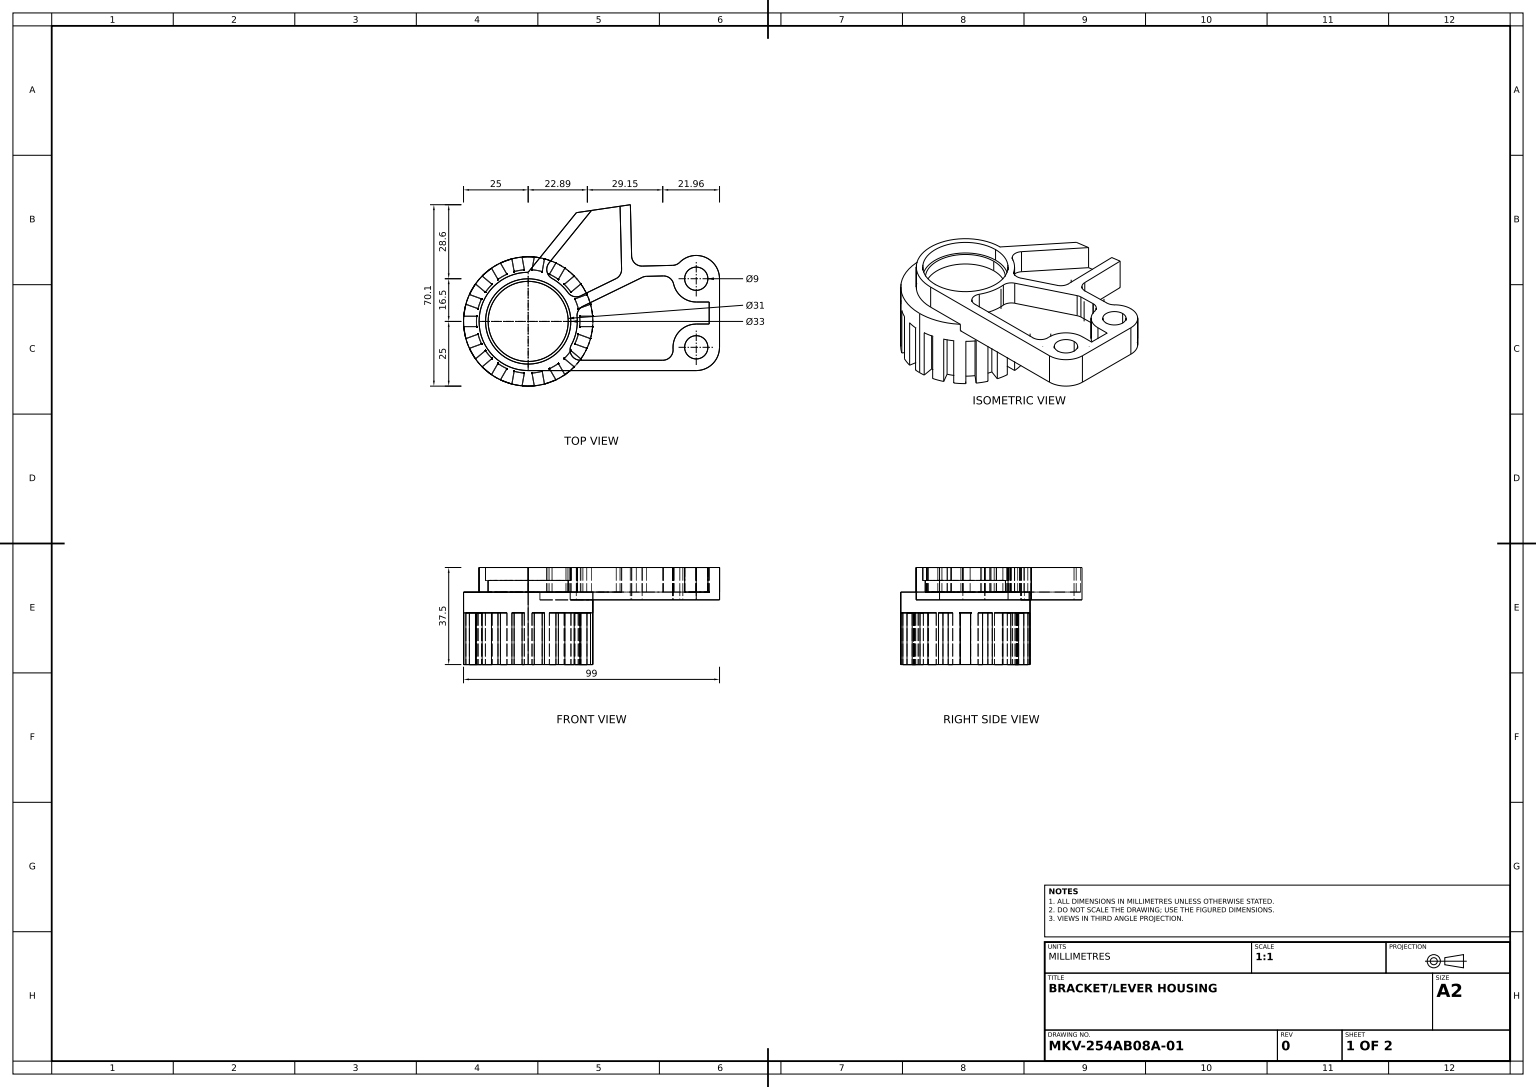
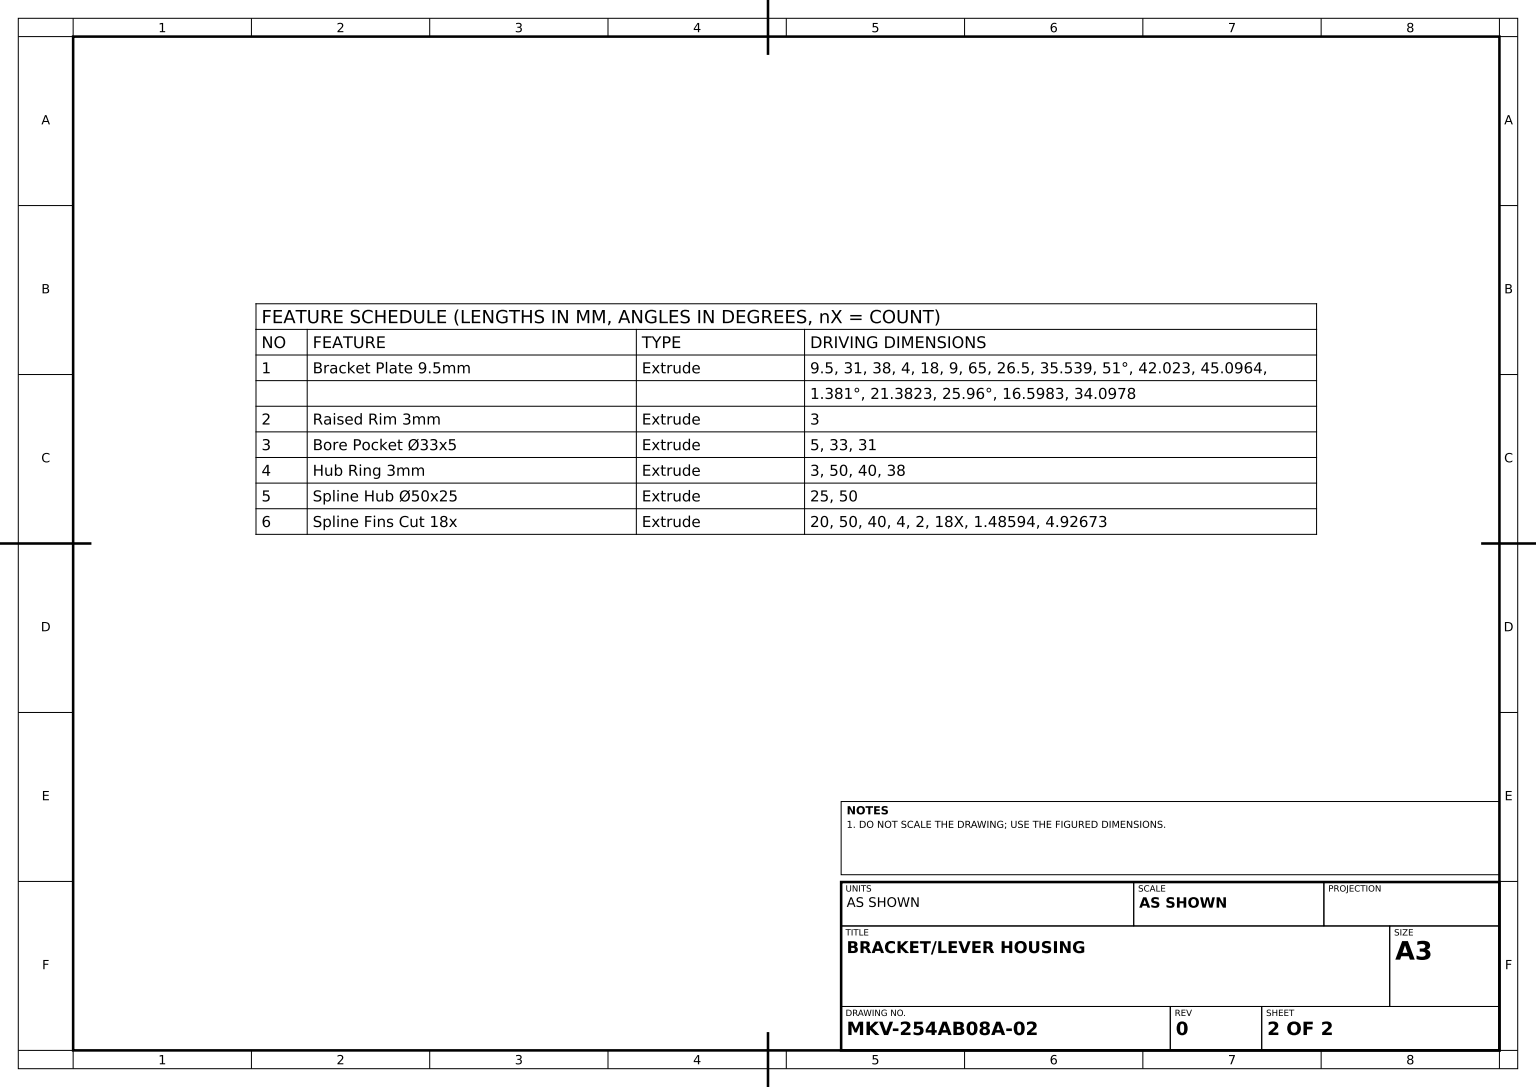
SolidWorks part; units mm, degrees
material "Plain Carbon Steel"
ref_plane "Front Plane" through (0, 0, 0) normal (0, 0, 1) x (1, 0, 0)
ref_plane "Top Plane" through (0, 0, 0) normal (0, 1, 0) x (1, 0, 0)
ref_plane "Right Plane" through (0, 0, 0) normal (1, 0, 0) x (0, 0, -1)
sketch "Bracket Plate Profile" plane through (0, 0, 0) normal (0, 1, 0) x (1, 0, 0)
  line L1 (0, 19) -> (18.6436, 42.023)
  line L3 (0, -19) -> (65, -19)
  line L4 (35.539, 44.5096) -> (36.1258, 20.1755)
  line L5 (44.099, 21.3823) -> (55.8769, 21.6663)
  line L6 (39.526, 45.0964) -> (40.0038, 25.2848)
  line L7 (8.0747, 22.6154) -> (24.4871, 42.883)
  line L8 (20.3648, 9.9133) -> (34.0978, 16.5983)
  line L9 (39.526, 45.0964) -> (18.6436, 42.023)
  line L10 (35.5272, 45) -> (36.2242, 16.0934) construction
  line L11 (74, 16.5) -> (74, -10)
  line L12 (39.526, 45.0964) -> (40.2231, 16.1898) construction
  line L13 (70, 7.5) -> (70, -1)
  line L14 (65, 7.5) -> (70, 7.5)
  line L15 (70, 7.5) -> (70, -1)
  line L16 (70, -1) -> (65, -1)
  line L17 (45.755, 17.4211) -> (52.2361, 17.5774)
  line L18 (70, 16.5) -> (70, -10) construction
  line L19 (20.199, -15) -> (52.0385, -15)
  line L21 (21.1394, 5.8416) -> (44.1007, 17.0188)
  line L23 (44.1954, 17.3835) -> (55.9733, 17.6675) construction
  line L24 (0, -15) -> (65, -15) construction
  circle A1 centre (0, 0) radius 15.5
  arc A2 (0, 19) -> (0, -19) centre (0, 0) ccw
  arc A3 (15.3769, 11.1603) -> (20.3648, 9.9133) centre (18.6141, 13.5098) ccw
  arc A4 (8.0747, 22.6154) -> (9.2384, 16.6028) centre (11.1833, 20.0981) ccw
  arc A5 (36.1258, 20.1755) -> (34.0978, 16.5983) centre (32.127, 20.079) cw
  arc A6 (74, 16.5) -> (58.6173, 22.8451) centre (65, 16.5) ccw
  circle A7 centre (65, 16.5) radius 4.5
  circle A8 centre (65, -10) radius 4.5
  arc A9 (65, -1) -> (56.0267, -10.6923) centre (65, -10) ccw
  arc A10 (44.099, 21.3823) -> (40.0038, 25.2848) centre (44.0026, 25.3812) cw
  arc A11 (58.6173, 22.8451) -> (55.8769, 21.6663) centre (55.7805, 25.6652) cw
  arc A12 (44.1007, 17.0188) -> (45.755, 17.4211) centre (45.8514, 13.4223) cw
  arc A13 (21.1394, 5.8416) -> (18.9093, 1.8546) centre (22.8902, 2.2451) ccw
  arc A14 (16.6861, -9.087) -> (20.199, -15) centre (20.199, -11) ccw
  arc A15 (56.0267, -10.6923) -> (52.0385, -15) centre (52.0385, -11) cw
  arc A16 (52.2361, 17.5774) -> (56.2302, 14.4775) centre (52.3325, 13.5786) cw
  arc A17 (65, -19) -> (74, -10) centre (65, -10) ccw
  arc A18 (56.2302, 14.4775) -> (65, 7.5) centre (65, 16.5) ccw
  arc A19 (15.3769, 11.1603) -> (9.2384, 16.6028) centre (0, 0) ccw
  arc A20 (16.6861, -9.087) -> (18.9093, 1.8546) centre (0, 0) ccw
  point P6 (3.1086, 16.4827)
  point P12 (9.4715, 24.3403)
  point P13 (3.1086, 16.4827)
  point P14 (21.7522, 39.5057)
  dimension "D1" = 31
  dimension "D2" = 38
  dimension "D3" = 51
  dimension "D6" = 4
  dimension "D7" = 4
  dimension "D8" = 4
  dimension "D4" = 18
  dimension "D5" = 9
  dimension "D12" = 26.5
  dimension "D14" = 4
  dimension "D15" = 4
  dimension "D19" = 4
  dimension "D21" = 4
  dimension "D22" = 4
  dimension "D23" = 4
  dimension "D24" = 4
  dimension "D26" = 9
  dimension "D27" = 9
  dimension "D9" = 4
  dimension "D11" = 65
  dimension "D13" = 9
  dimension "D16" = 4
  dimension "D17" = 4
  dimension "D18" = 35.539
  dimension "D20" = 4
  dimension "D25" = 4
  dimension "D28" = 42.023
  dimension "D29" = 45.0964
  dimension "D30" = 1.381
  dimension "D31" = 21.3823
  dimension "D32" = 25.956
  dimension "D33" = 16.5983
  dimension "D34" = 34.0978
  dimension "D10" = 4
extrude "Bracket Plate 9.5mm" add sketch "Bracket Plate Profile" along normal blind 9.5 contours A3 A19 A4 L7 L9 L1 A2 L3 A17 L11 A6 A11 L5 A10 L6 L4 A5 L8 A1 A7 A8 A14 A20 A13 L21 A12 L17 A16 A18 L14 L13 L16 A9 A15 L19
sketch "Raised Rim Profile" plane through (0, 0, 0) normal (0, -1, 0) x (1, 0, 0)
  line L0 (0, 19) -> (65, 19)
  line L1 (74, 10) -> (74, -16.5)
  line L2 (55.8769, -21.6663) -> (44.099, -21.3823)
  line L3 (40.0038, -25.2848) -> (39.526, -45.0964)
  line L4 (39.526, -45.0964) -> (18.6436, -42.023)
  line L5 (18.6436, -42.023) -> (0, -19)
  circle A0 centre (0, 0) radius 19
  arc A1 (65, 19) -> (74, 10) centre (65, 10) cw
  arc A2 (74, -16.5) -> (58.6173, -22.8451) centre (65, -16.5) cw
  arc A3 (55.8769, -21.6663) -> (58.6173, -22.8451) centre (55.7805, -25.6652) cw
  arc A4 (44.099, -21.3823) -> (40.0038, -25.2848) centre (44.0026, -25.3812) ccw
  circle M1 centre (0, 0) radius 15.5
  circle M2 centre (65, -16.5) radius 4.5
  circle M3 centre (65, 10) radius 4.5
  arc M4 (15.3769, -11.1603) -> (20.3648, -9.9133) centre (18.6141, -13.5098) cw
  line M5 (20.3648, -9.9133) -> (34.0978, -16.5983)
  arc M6 (34.0978, -16.5983) -> (36.1258, -20.1755) centre (32.127, -20.079) cw
  line M7 (36.1258, -20.1755) -> (35.539, -44.5096)
  line M8 (35.539, -44.5096) -> (39.526, -45.0964)
  line M9 (39.526, -45.0964) -> (40.0038, -25.2848)
  arc M10 (40.0038, -25.2848) -> (44.099, -21.3823) centre (44.0026, -25.3812) cw
  line M11 (44.099, -21.3823) -> (55.8769, -21.6663)
  arc M12 (55.8769, -21.6663) -> (58.6173, -22.8451) centre (55.7805, -25.6652) cw
  arc M13 (58.6173, -22.8451) -> (74, -16.5) centre (65, -16.5) ccw
  line M14 (74, -16.5) -> (74, 10)
  arc M15 (74, 10) -> (65, 19) centre (65, 10) ccw
  line M16 (65, 19) -> (0, 19)
  arc M17 (0, 19) -> (0, -19) centre (0, 0) ccw
  line M18 (0, -19) -> (18.6436, -42.023)
  line M19 (18.6436, -42.023) -> (24.4871, -42.883)
  line M20 (24.4871, -42.883) -> (8.0747, -22.6154)
  arc M21 (8.0747, -22.6154) -> (9.2384, -16.6028) centre (11.1833, -20.0981) cw
  arc M22 (9.2384, -16.6028) -> (15.3769, -11.1603) centre (0, 0) ccw
  arc M23 (16.6861, 9.087) -> (20.199, 15) centre (20.199, 11) cw
  line M24 (20.199, 15) -> (52.0385, 15)
  arc M25 (52.0385, 15) -> (56.0267, 10.6923) centre (52.0385, 11) cw
  arc M26 (56.0267, 10.6923) -> (65, 1) centre (65, 10) ccw
  line M27 (65, 1) -> (70, 1)
  line M28 (70, 1) -> (70, -7.5)
  line M29 (70, -7.5) -> (65, -7.5)
  arc M30 (65, -7.5) -> (56.2302, -14.4775) centre (65, -16.5) ccw
  arc M31 (56.2302, -14.4775) -> (52.2361, -17.5774) centre (52.3325, -13.5786) cw
  line M32 (52.2361, -17.5774) -> (45.755, -17.4211)
  arc M33 (45.755, -17.4211) -> (44.1007, -17.0188) centre (45.8514, -13.4223) cw
  line M34 (44.1007, -17.0188) -> (21.1394, -5.8416)
  arc M35 (21.1394, -5.8416) -> (18.9093, -1.8546) centre (22.8902, -2.2451) cw
  arc M36 (18.9093, -1.8546) -> (16.6861, 9.087) centre (0, 0) ccw
extrude "Raised Rim 3mm" add sketch "Raised Rim Profile" along normal blind 3 contours A0 M17 M22 M36 M1 | M1 | A0 M4 M5 M6 M7 M8 M9 M10 M11 M12 M13 M14 M15 M16 M23 M24 M25 M26 M27 M28 M29 M30 M31 M32 M33 M34 M35 M2 M3 | M3 | M2 | M23 M36 M35 M34 M33 M32 M31 M30 M29 M28 M27 M26 M25 M24 | L4 M7 M6 M5 M4 M22 M21 M20 | A0 M18 M19 M20 M21
sketch "Bore Pocket Profile" plane through (0, 9.5, 0) normal (0, 1, 0) x (1, 0, 0)
  circle A0 centre (0, 0) radius 16.5
  circle A1 centre (0, 0) radius 15.5
  dimension "D1" = 33
  dimension "D2" = 31
extrude "Bore Pocket Ø33x5" cut sketch "Bore Pocket Profile" against normal blind 5
sketch "Hub Ring Profile" plane through (0, -3, 0) normal (0, -1, 0) x (1, 0, 0)
  circle A0 centre (0, 0) radius 25
  circle A1 centre (0, 0) radius 20
  circle A2 centre (0, 0) radius 19
  line M9 (65, 19) -> (0, 19)
  arc M10 (0, 19) -> (0, -19) centre (0, 0) ccw
  line M11 (0, -19) -> (18.6436, -42.023)
  dimension "D1" = 50
  dimension "D2" = 40
  dimension "D3" = 38
extrude "Hub Ring 3mm" add sketch "Hub Ring Profile" against normal blind 3 contours A1 M9 M11 M10 | A1 A0 M9 M11
sketch "Hub Profile Ø50" plane through (0, -3, 0) normal (0, -1, 0) x (1, 0, 0)
  circle A0 centre (0, 0) radius 25
  dimension "D1" = 50
extrude "Spline Hub Ø50x25" add sketch "Hub Profile Ø50" along normal blind 25
sketch "Spline Fin Profile 18x" plane through (0, -28, 0) normal (0, -1, 0) x (1, 0, 0)
  line L0 (19.3837, -4.9267) -> (24.1011, -6.6437)
  line L1 (19.8997, -2) -> (24.9199, -2)
  line L2 (19.8997, 2) -> (24.9199, 2)
  line L3 (18.0156, -8.6855) -> (22.733, -10.4025)
  line L4 (16.5297, -11.2592) -> (20.3753, -14.4861)
  line L5 (13.9585, -14.3234) -> (17.8042, -17.5503)
  line L6 (11.6819, -16.2337) -> (14.192, -20.5812)
  line L7 (8.2178, -18.2337) -> (10.7279, -22.5812)
  line L8 (5.4252, -19.2501) -> (6.2969, -24.194)
  line L9 (1.4859, -19.9447) -> (2.3577, -24.8886)
  line L10 (-1.4859, -19.9447) -> (-2.3577, -24.8886)
  line L11 (-5.4252, -19.2501) -> (-6.2969, -24.194)
  line L12 (-8.2178, -18.2337) -> (-10.7279, -22.5812)
  line L13 (-11.6819, -16.2337) -> (-14.192, -20.5812)
  line L14 (-13.9585, -14.3234) -> (-17.8042, -17.5503)
  line L15 (-16.5297, -11.2592) -> (-20.3753, -14.4861)
  line L16 (-18.0156, -8.6855) -> (-22.733, -10.4025)
  line L17 (-19.3837, -4.9267) -> (-24.1011, -6.6437)
  line L18 (-19.8997, -2) -> (-24.9199, -2)
  line L19 (-19.8997, 2) -> (-24.9199, 2)
  line L20 (-19.3837, 4.9267) -> (-24.1011, 6.6437)
  line L21 (-18.0156, 8.6855) -> (-22.733, 10.4025)
  line L22 (-16.5297, 11.2592) -> (-20.3753, 14.4861)
  line L23 (-13.9585, 14.3234) -> (-17.8042, 17.5503)
  line L24 (-11.6819, 16.2337) -> (-14.192, 20.5812)
  line L25 (-8.2178, 18.2337) -> (-10.7279, 22.5812)
  line L26 (-5.4252, 19.2501) -> (-6.2969, 24.194)
  line L27 (-1.4859, 19.9447) -> (-2.3577, 24.8886)
  line L28 (1.4859, 19.9447) -> (2.3577, 24.8886)
  line L29 (5.4252, 19.2501) -> (6.2969, 24.194)
  line L30 (8.2178, 18.2337) -> (10.7279, 22.5812)
  line L31 (11.6819, 16.2337) -> (14.192, 20.5812)
  line L32 (13.9585, 14.3234) -> (17.8042, 17.5503)
  line L33 (16.5297, 11.2592) -> (20.3753, 14.4861)
  line L34 (18.0156, 8.6855) -> (22.733, 10.4025)
  line L35 (19.3837, 4.9267) -> (24.1011, 6.6437)
  circle A0 centre (0, 0) radius 25
  arc A1 (19.8997, -2) -> (19.8997, 2) centre (0, 0) ccw
  arc A2 (19.3837, 4.9267) -> (18.0156, 8.6855) centre (0, 0) ccw
  arc A3 (19.8997, -2) -> (19.8997, 2) centre (0, 0) ccw
  arc A4 (18.0156, -8.6855) -> (19.3837, -4.9267) centre (0, 0) ccw
  arc A5 (13.9585, -14.3234) -> (16.5297, -11.2592) centre (0, 0) ccw
  arc A6 (8.2178, -18.2337) -> (11.6819, -16.2337) centre (0, 0) ccw
  arc A7 (1.4859, -19.9447) -> (5.4252, -19.2501) centre (0, 0) ccw
  arc A8 (-5.4252, -19.2501) -> (-1.4859, -19.9447) centre (0, 0) ccw
  arc A9 (-11.6819, -16.2337) -> (-8.2178, -18.2337) centre (0, 0) ccw
  arc A10 (-16.5297, -11.2592) -> (-13.9585, -14.3234) centre (0, 0) ccw
  arc A11 (-19.3837, -4.9267) -> (-18.0156, -8.6855) centre (0, 0) ccw
  arc A12 (-19.8997, 2) -> (-19.8997, -2) centre (0, 0) ccw
  arc A13 (-18.0156, 8.6855) -> (-19.3837, 4.9267) centre (0, 0) ccw
  arc A14 (-13.9585, 14.3234) -> (-16.5297, 11.2592) centre (0, 0) ccw
  arc A15 (-8.2178, 18.2337) -> (-11.6819, 16.2337) centre (0, 0) ccw
  arc A16 (-1.4859, 19.9447) -> (-5.4252, 19.2501) centre (0, 0) ccw
  arc A17 (5.4252, 19.2501) -> (1.4859, 19.9447) centre (0, 0) ccw
  arc A18 (11.6819, 16.2337) -> (8.2178, 18.2337) centre (0, 0) ccw
  arc A19 (16.5297, 11.2592) -> (13.9585, 14.3234) centre (0, 0) ccw
  circle A20 centre (0, 0) radius 25 construction
  point P4 (0, -3)
  point P5 (25, 0)
  point P6 (25, -3)
  point P7 (0, 3)
  point P8 (25, 3)
  circle M4 centre (0, 0) radius 25
  dimension "D1" = 50
  dimension "D2" = 40
  dimension "D4" = 2
  dimension "D5" = 1.4859
  dimension "D3" = 4
  dimension "D7" = 4.9267
  dimension "D6" = 18
extrude "Spline Fins Cut 18x" cut sketch "Spline Fin Profile 18x" against normal blind 20 contours A12 L19 L18 M4 | A11 L17 L16 M4 | A10 L15 L14 M4 | A9 L13 L12 M4 | A8 L11 L10 M4 | A7 L9 L8 M4 | A6 L7 L6 M4 | A5 L5 L4 M4 | A4 L3 L0 M4 | A1 L1 L2 M4 | A2 L35 L34 M4 | A19 L33 L32 M4 | A18 L31 L30 M4 | A17 L29 L28 M4 | A16 L27 L26 M4 | A15 L25 L24 M4 | A14 L23 L22 M4 | A13 L21 L20 M4
